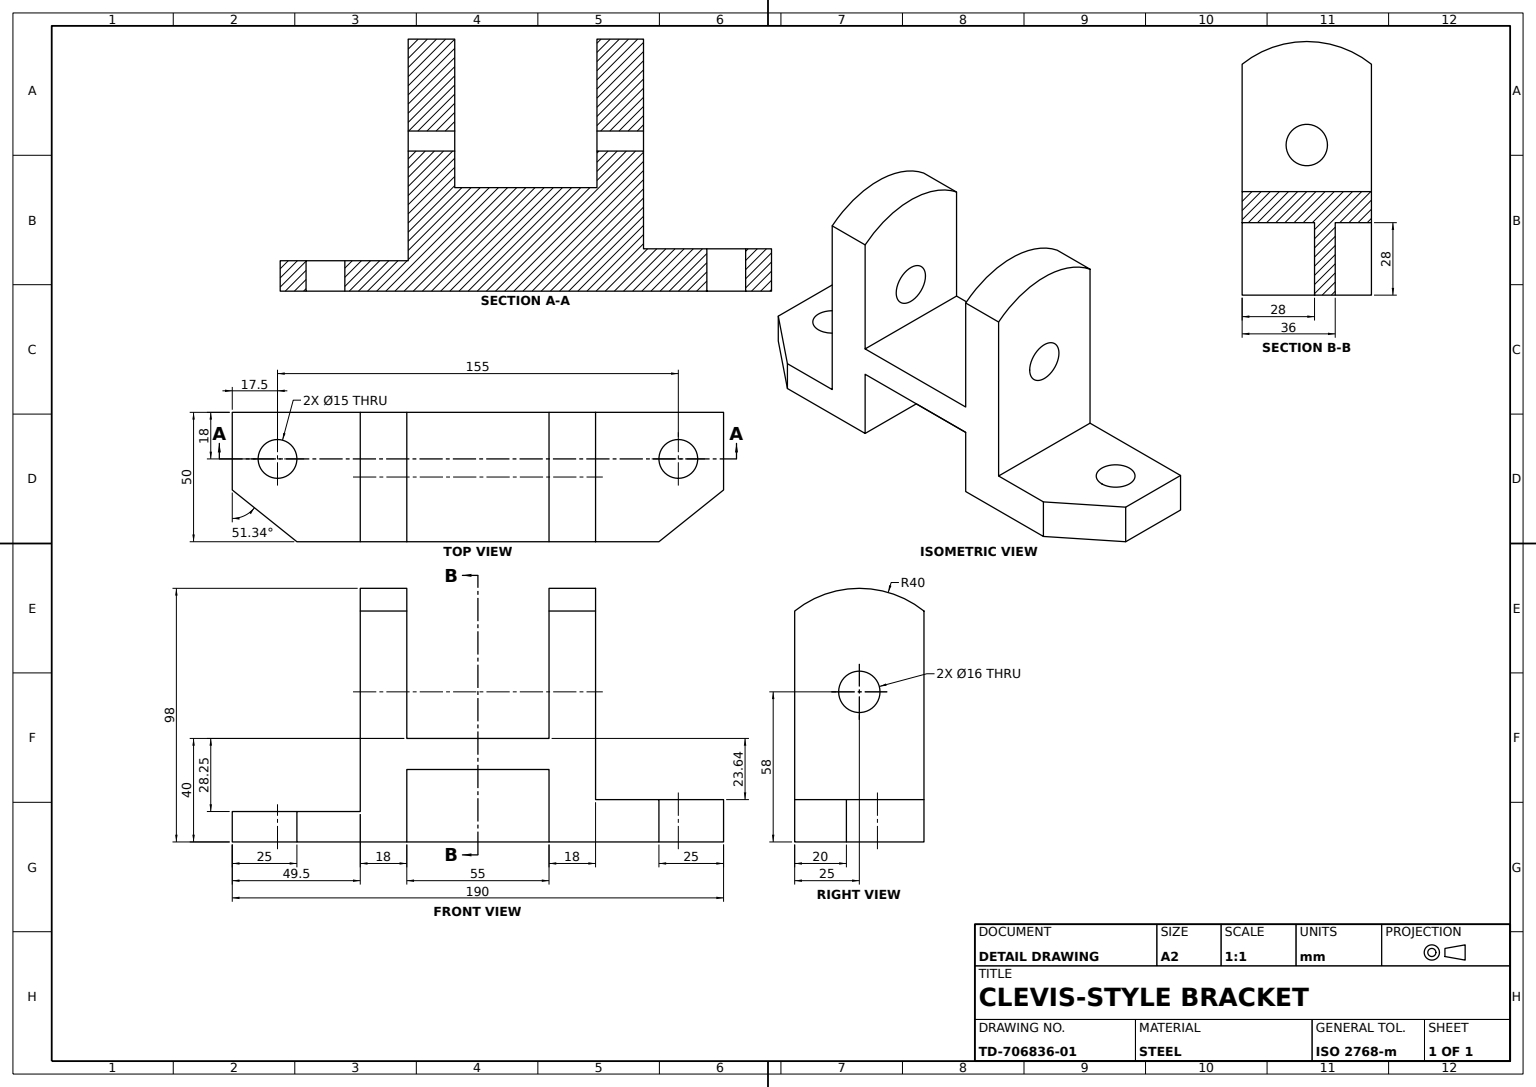
SolidWorks part; units mm, degrees
material "Plain Carbon Steel"
ref_plane "Front Plane" through (0, 0, 0) normal (0, 0, 1) x (1, 0, 0)
ref_plane "Top Plane" through (0, 0, 0) normal (0, 1, 0) x (1, 0, 0)
ref_plane "Right Plane" through (0, 0, 0) normal (1, 0, 0) x (0, 0, -1)
sketch "Bracket Side Profile Sketch" plane through (0, 0, 0) normal (0, 0, 1) x (1, 0, 0)
  line L0 (-95, -28.2452) -> (-95, -40)
  line L1 (-95, -40) -> (95, -40)
  line L2 (95, -40) -> (95, -23.6423)
  line L3 (95, -23.6423) -> (45.5, -23.6423)
  line L4 (45.5, -23.6423) -> (45.5, 58)
  line L5 (45.5, 58) -> (27.5, 58)
  line L6 (27.5, 58) -> (27.5, 0)
  line L7 (27.5, 0) -> (-27.5, 0)
  line L8 (-27.5, 0) -> (-27.5, 58)
  line L9 (-27.5, 58) -> (-45.5, 58)
  line L10 (-45.5, 58) -> (-45.5, -28.2452)
  line L11 (-45.5, -28.2452) -> (-95, -28.2452)
  point P13 (-36.5, 58)
  dimension "D1" = 190
  dimension "D2" = 55
  dimension "D3" = 27.5
  dimension "D4" = 18
  dimension "D5" = 18
  dimension "D6" = 58
  dimension "D7" = 58
  dimension "D8" = 40
  dimension "D9" = 49.5
  dimension "D10" = 28.2452
  dimension "D11" = 23.6423
extrude "Bracket Body" add sketch "Bracket Side Profile Sketch" along normal mid plane 50
sketch "Upright Rounds and Pin Hole Sketch" plane through (45.5, 0, 0) normal (1, 0, 0) x (0, 0, -1)
  line L0 (-25, 58) -> (25, 58) construction
  line L1 (-25, 49.225) -> (-25, 58)
  line L4 (25, 58) -> (25, 49.225)
  line L6 (-25, 49.225) -> (-25, 66.8008)
  line L7 (-25, 66.8008) -> (25, 66.8008)
  line L8 (25, 66.8008) -> (25, 49.225)
  circle A0 centre (0, 18) radius 8
  arc A1 (25, 49.225) -> (-25, 49.225) centre (0, 18) ccw
  line M1 (25, -23.6423) -> (25, 58)
  line M2 (25, 58) -> (-25, 58)
  line M3 (-25, 58) -> (-25, -23.6423)
  dimension "D1" = 16
  dimension "D2" = 80
  dimension "D3" = 40
  dimension "D4" = 8.8008
extrude "Upright Rounds and Pin Hole Ø16" cut sketch "Upright Rounds and Pin Hole Sketch" against normal blind 120 contours A1 M2 M3 | L8 L7 L6 M2 | A1 M1 M2 | A0
chamfer "Flange Corner Chamfers" distance 20 distance2 25 2 edges at (-95, -34.1226, 25) (95, -31.8211, 25)
sketch "Mounting Holes and Relief Sketch" plane through (0, -40, 0) normal (0, -1, 0) x (1, 0, 0)
  line L0 (-95, -25) -> (95, -25) construction
  line L2 (-70, 25) -> (70, 25) construction
  line L3 (-27.5, 25) -> (27.5, 25)
  line L4 (-27.5, 25) -> (-27.5, -3)
  line L5 (-27.5, -25) -> (27.5, -25)
  line L6 (27.5, 25) -> (27.5, -3)
  line L9 (-27.5, -3) -> (27.5, -3)
  line L11 (-27.5, -11) -> (-27.5, -25)
  line L13 (-27.5, -11) -> (27.5, -11)
  line L18 (27.5, -11) -> (27.5, -25)
  circle A0 centre (-77.5, -7) radius 7.5
  circle A1 centre (77.5, -7) radius 7.5
  dimension "D1" = 15
  dimension "D2" = 15
  dimension "D3" = 155
  dimension "D4" = 18
  dimension "D5" = 77.5
  dimension "D6" = 55
  dimension "D7" = 27.5
  dimension "D8" = 28
  dimension "D9" = 36
extrude "Mounting Holes 2xØ15 and Centre Relief" cut sketch "Mounting Holes and Relief Sketch" against normal blind 28
